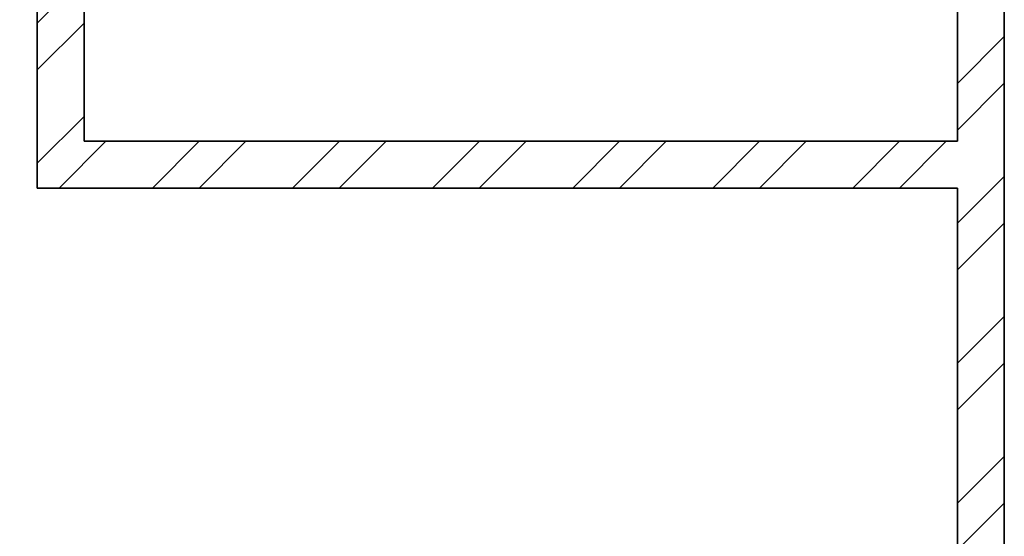
# Model space of a CAD drawing. Units: inches. Extents: x 1885 to 2748, y 783 to 2421.
# Tile 110 of 117: x 2524 to 2618, y 1977 to 2027. Entities that reach past the tile are written whole.
import ezdxf

# ---------------------------------------------------------------- set-up
doc = ezdxf.new("R2010")
doc.units = ezdxf.units.IN
doc.layers.add('A-WALL', color=7, linetype='Continuous', lineweight=35)
doc.layers.add('A-WALL-PATT', color=85, linetype='Continuous', lineweight=13, true_color=0x58ba48)

msp = doc.modelspace()

# ---------------------------------------------------------------- hatches: boundary and pattern name
at = {"layer": 'A-WALL-PATT'}
h = msp.add_hatch(dxfattribs=at)
h.set_pattern_fill('ANSI32', color=256)
h.paths.add_polyline_path([(2007.772, 2318.006), (1980.774, 2318.006), (1980.774, 2281.215), (1985.274, 2281.215), (1985.274, 2313.506), (2007.772, 2313.506), (2007.772, 2315.756)])
h.paths.add_polyline_path([(2094.324, 2318.006), (2067.772, 2318.006), (2067.772, 2313.506), (2094.324, 2313.506), (2094.324, 2315.756)])
h.paths.add_polyline_path([(2131.367, 2315.756), (2131.367, 2318.006), (2131.189, 2318.006), (2112.609, 2318.006), (2112.609, 2313.506), (2117.274, 2313.506), (2117.274, 2255.201), (2121.774, 2255.201), (2121.774, 2313.506), (2131.367, 2313.506)])
h.paths.add_polyline_path([(2190.512, 2318.006), (2155.367, 2318.006), (2155.367, 2313.506), (2169.774, 2313.506), (2169.774, 2229.506), (2121.774, 2229.506), (2121.774, 2233.451), (2119.524, 2233.451), (2117.274, 2233.451), (2117.274, 2201.101), (2121.774, 2201.101), (2121.774, 2225.006), (2169.774, 2225.006), (2169.774, 2165.006), (2306.274, 2165.006), (2306.274, 2066.006), (2310.774, 2066.006), (2344.274, 2066.006), (2486.274, 2066.006), (2486.274, 1886.006), (2483.02, 1886.006), (2483.02, 1881.506), (2486.274, 1881.506), (2486.274, 1880.678), (2490.774, 1880.678), (2490.774, 2070.506), (2344.274, 2070.506), (2310.774, 2070.506), (2310.774, 2165.006), (2310.774, 2173.636), (2308.524, 2173.636), (2306.274, 2173.636), (2306.274, 2169.506), (2174.274, 2169.506), (2174.274, 2313.506), (2190.512, 2313.506), (2190.512, 2315.756)])
h.paths.add_polyline_path([(1985.274, 2221.215), (1980.774, 2221.215), (1980.774, 2165.006), (1992.774, 2165.006), (1992.774, 2141.927), (1997.274, 2141.927), (1997.274, 2165.006), (2117.274, 2165.006), (2117.274, 2163.126), (2121.774, 2163.126), (2121.774, 2172.734), (2119.524, 2172.734), (2117.274, 2172.734), (2117.274, 2169.506), (1985.274, 2169.506)])
h.paths.add_polyline_path([(1997.274, 2105.927), (1992.774, 2105.927), (1992.774, 2070.506), (2016.774, 2070.506), (2016.774, 2059.123), (2019.024, 2059.123), (2021.274, 2059.123), (2021.274, 2070.506), (2117.274, 2070.506), (2117.274, 2022.506), (2114.423, 2022.506), (2114.423, 2018.006), (2123.627, 2018.006), (2123.627, 2020.256), (2123.627, 2022.506), (2121.774, 2022.506), (2121.774, 2142.587), (2119.524, 2142.587), (2117.274, 2142.587), (2117.274, 2075.006), (1997.274, 2075.006)])
h.paths.add_polyline_path([(2092.029, 2020.256), (2092.029, 2022.506), (2021.274, 2022.506), (2021.274, 2035.123), (2016.774, 2035.123), (2016.774, 2018.006), (2016.774, 1978.784), (2021.274, 1978.784), (2021.274, 2018.006), (2092.029, 2018.006)])
h.paths.add_polyline_path([(2260.938, 2022.506), (2153.105, 2022.506), (2153.105, 2020.256), (2153.105, 2018.006), (2155.274, 2018.006), (2155.274, 1886.006), (2107.629, 1886.006), (2107.629, 1881.506), (2182.911, 1881.506), (2182.911, 1883.756), (2182.911, 1886.006), (2159.774, 1886.006), (2159.774, 2018.006), (2260.938, 2018.006), (2260.938, 2020.256)])
h.paths.add_polyline_path([(2047.629, 1883.756), (2047.629, 1886.006), (2021.274, 1886.006), (2021.274, 1918.784), (2019.024, 1918.784), (2016.774, 1918.784), (2016.774, 1881.506), (2047.629, 1881.506)])
h.paths.add_polyline_path([(2306.361, 1883.756), (2306.361, 1886.006), (2296.274, 1886.006), (2296.274, 1982.006), (2316.535, 1982.006), (2316.535, 1984.256), (2316.535, 1986.506), (2296.274, 1986.506), (2296.274, 2022.506), (2289.276, 2022.506), (2289.276, 2018.006), (2291.774, 2018.006), (2291.774, 1886.006), (2242.911, 1886.006), (2242.911, 1881.506), (2306.361, 1881.506)], flags=17)
h.paths.add_polyline_path([(1985.274, 1843.006), (2021.6, 1843.006), (2021.534, 1845.441), (2021.477, 1847.506), (1980.774, 1847.506), (1980.774, 1809.446), (1985.274, 1809.446)])
h.paths.add_polyline_path([(2131.482, 1845.256), (2131.482, 1847.506), (2081.534, 1847.506), (2081.534, 1843.006), (2117.274, 1843.006), (2117.274, 1784.147), (2119.524, 1784.147), (2121.774, 1784.147), (2121.774, 1843.006), (2131.482, 1843.006)])
h.paths.add_polyline_path([(2203.886, 1847.506), (2155.482, 1847.506), (2155.482, 1843.006), (2169.774, 1843.006), (2169.774, 1759.006), (2121.774, 1759.006), (2121.774, 1761.457), (2117.274, 1761.457), (2117.274, 1730.429), (2121.774, 1730.429), (2121.774, 1754.506), (2177.421, 1754.506), (2177.421, 1756.756), (2177.421, 1759.006), (2174.274, 1759.006), (2174.274, 1843.006), (2203.886, 1843.006)])
h.paths.add_polyline_path([(2335.554, 1845.256), (2335.554, 1847.506), (2239.886, 1847.506), (2239.886, 1843.006), (2306.274, 1843.006), (2306.274, 1759.006), (2199.486, 1759.006), (2199.486, 1754.506), (2310.774, 1754.506), (2310.774, 1843.006), (2335.554, 1843.006)])
h.paths.add_polyline_path([(2348.774, 2022.506), (2344.274, 2022.506), (2344.274, 1986.506), (2341.681, 1986.506), (2341.681, 1982.006), (2344.274, 1982.006), (2344.274, 1886.006), (2330.361, 1886.006), (2330.361, 1881.506), (2361.627, 1881.506), (2361.627, 1883.756), (2361.627, 1886.006), (2348.774, 1886.006)], flags=17)
h.paths.add_polyline_path([(2283.251, 2315.756), (2283.251, 2318.006), (2238.512, 2318.006), (2238.512, 2313.506), (2283.251, 2313.506)], flags=17)
h.paths.add_polyline_path([(2363.274, 2348.006), (2388.677, 2348.006), (2388.677, 2350.256), (2388.677, 2352.506), (2358.774, 2352.506), (2358.774, 2348.006), (2358.774, 2318.006), (2344.481, 2318.006), (2344.481, 2313.506), (2358.774, 2313.506), (2358.774, 2229.506), (2310.774, 2229.506), (2310.774, 2231.952), (2306.274, 2231.952), (2306.274, 2205.611), (2310.774, 2205.611), (2310.774, 2225.006), (2358.774, 2225.006), (2358.774, 2211.506), (2452.329, 2211.506), (2452.329, 2213.756), (2452.329, 2216.006), (2363.274, 2216.006), (2363.274, 2318.006)])
h.paths.add_polyline_path([(2310.774, 2313.506), (2320.481, 2313.506), (2320.481, 2315.756), (2320.481, 2318.006), (2302.728, 2318.006), (2302.728, 2313.506), (2306.274, 2313.506), (2306.274, 2251.076), (2310.774, 2251.076)], flags=17)
h.paths.add_polyline_path([(2490.774, 2352.506), (2486.274, 2352.506), (2448.677, 2352.506), (2448.677, 2348.006), (2486.274, 2348.006), (2486.274, 2318.006), (2486.274, 2216.006), (2481.78, 2216.006), (2481.78, 2211.506), (2486.274, 2211.506), (2486.274, 2165.006), (2493.289, 2165.006), (2493.289, 2167.256), (2493.289, 2169.506), (2490.774, 2169.506), (2490.774, 2313.506), (2494.429, 2313.506), (2494.429, 2318.006), (2490.774, 2318.006)])
h.paths.add_polyline_path([(2534.653, 2318.006), (2515.691, 2318.006), (2515.691, 2313.506), (2534.653, 2313.506), (2534.653, 2315.756)])
h.paths.add_polyline_path([(2618.274, 2318.006), (2594.653, 2318.006), (2594.653, 2313.506), (2613.774, 2313.506), (2613.774, 2281.706), (2618.274, 2281.706)])
h.paths.add_polyline_path([(2618.274, 2221.706), (2613.774, 2221.706), (2613.774, 2169.506), (2554.019, 2169.506), (2554.019, 2165.006), (2613.774, 2165.006), (2613.774, 2152.878), (2618.274, 2152.878)])
h.paths.add_polyline_path([(2618.274, 2128.878), (2616.024, 2128.878), (2613.774, 2128.878), (2613.774, 2117.006), (2529.774, 2117.006), (2529.774, 2165.006), (2532.848, 2165.006), (2532.848, 2169.506), (2522.867, 2169.506), (2522.867, 2165.006), (2525.274, 2165.006), (2525.274, 2117.006), (2525.274, 2112.506), (2525.274, 2108.576), (2529.774, 2108.576), (2529.774, 2112.506), (2613.774, 2112.506), (2613.774, 2080.19), (2618.274, 2080.19)])
h.paths.add_polyline_path([(2618.274, 2044.19), (2616.024, 2044.19), (2613.774, 2044.19), (2613.774, 2015.506), (2529.774, 2015.506), (2529.774, 2088.582), (2527.524, 2088.582), (2525.274, 2088.582), (2525.274, 2011.006), (2613.774, 2011.006), (2613.774, 1956.755), (2618.274, 1956.755)])
h.paths.add_polyline_path([(2618.274, 1881.506), (2618.274, 1896.755), (2613.774, 1896.755), (2613.774, 1881.506), (2613.774, 1847.506), (2592.715, 1847.506), (2592.715, 1843.006), (2613.774, 1843.006), (2613.774, 1765.006), (2613.774, 1760.506), (2609.621, 1760.506), (2609.621, 1756.006), (2613.774, 1756.006), (2613.774, 1660.006), (2608.544, 1660.006), (2608.544, 1655.506), (2613.774, 1655.506), (2613.774, 1508.158), (2618.274, 1508.158)])
h.paths.add_polyline_path([(2565.774, 1843.006), (2568.997, 1843.006), (2568.997, 1847.506), (2490.774, 1847.506), (2490.774, 1849.7), (2488.524, 1849.7), (2486.274, 1849.7), (2486.274, 1847.506), (2477.274, 1847.506), (2477.274, 1838.506), (2477.274, 1821.493), (2486.274, 1821.493), (2486.274, 1838.506), (2561.274, 1838.506), (2561.274, 1765.006), (2486.274, 1765.006), (2486.274, 1786.157), (2477.274, 1786.157), (2477.274, 1765.006), (2477.274, 1756.006), (2486.274, 1756.006), (2565.774, 1756.006), (2585.621, 1756.006), (2585.621, 1758.256), (2585.621, 1760.506), (2565.774, 1760.506), (2565.774, 1765.006)])
h.paths.add_polyline_path([(2486.274, 1651.006), (2561.274, 1651.006), (2561.274, 1567.006), (2486.274, 1567.006), (2486.274, 1591.321), (2477.274, 1591.321), (2477.274, 1567.006), (2477.274, 1558.006), (2477.274, 1555.439), (2481.774, 1555.439), (2481.774, 1558.006), (2568.653, 1558.006), (2568.653, 1560.256), (2568.653, 1562.506), (2565.774, 1562.506), (2565.774, 1655.506), (2584.544, 1655.506), (2584.544, 1657.756), (2584.544, 1660.006), (2565.774, 1660.006), (2486.274, 1660.006), (2477.274, 1660.006), (2477.274, 1651.006), (2477.274, 1632.989), (2486.274, 1632.989)])
h.paths.add_polyline_path([(2449.967, 1883.756), (2449.967, 1886.006), (2421.627, 1886.006), (2421.627, 1881.506), (2449.967, 1881.506)], flags=17)
h.paths.add_polyline_path([(2447.274, 1847.506), (2395.554, 1847.506), (2395.554, 1843.006), (2442.774, 1843.006), (2442.774, 1809.27), (2447.274, 1809.27)])
h.paths.add_polyline_path([(1985.274, 1749.446), (1980.774, 1749.446), (1980.774, 1694.504), (1985.274, 1694.504), (1985.274, 1694.506), (1986.897, 1694.506), (1986.897, 1697.78), (1986.897, 1699.006), (1985.274, 1699.006)])
h.paths.add_polyline_path([(2152.774, 1699.006), (2121.774, 1699.006), (2121.774, 1703.668), (2119.524, 1703.668), (2117.274, 1703.668), (2117.274, 1699.006), (2009.219, 1699.006), (2009.219, 1694.506), (2148.274, 1694.506), (2148.274, 1692.631), (2152.774, 1692.631)])
h.paths.add_polyline_path([(2016.274, 1694.506), (2011.774, 1694.506), (2011.774, 1558.006), (2040.806, 1558.006), (2040.806, 1560.256), (2040.806, 1562.506), (2016.274, 1562.506)])
h.paths.add_polyline_path([(2152.774, 1663.017), (2150.524, 1663.017), (2148.274, 1663.017), (2148.274, 1562.506), (2100.806, 1562.506), (2100.806, 1558.006), (2165.119, 1558.006), (2165.119, 1560.256), (2165.119, 1562.506), (2152.774, 1562.506), (2152.774, 1610.506), (2224.774, 1610.506), (2224.774, 1607.99), (2229.274, 1607.99), (2229.274, 1615.006), (2152.774, 1615.006)])
h.paths.add_polyline_path([(2238.613, 1560.256), (2238.613, 1562.506), (2229.274, 1562.506), (2229.274, 1588.756), (2227.024, 1588.763), (2224.774, 1588.771), (2224.774, 1562.506), (2189.119, 1562.506), (2189.119, 1558.006), (2238.613, 1558.006)])
h.paths.add_polyline_path([(2336.024, 1560.256), (2336.024, 1562.506), (2310.774, 1562.506), (2310.774, 1656.347), (2308.524, 1656.347), (2306.274, 1656.347), (2306.274, 1562.506), (2286.613, 1562.506), (2286.613, 1558.006), (2336.024, 1558.006)])
h.paths.add_polyline_path([(2447.274, 1690.968), (2445.024, 1690.968), (2442.774, 1690.968), (2442.774, 1687.006), (2306.274, 1687.006), (2306.274, 1680.75), (2310.774, 1680.75), (2310.774, 1682.506), (2442.774, 1682.506), (2442.774, 1562.506), (2396.024, 1562.506), (2396.024, 1558.006), (2447.274, 1558.006)])
h.paths.add_polyline_path([(2447.274, 1749.27), (2445.024, 1749.27), (2442.774, 1749.27), (2442.774, 1717.232), (2447.274, 1717.232)])
h.paths.add_polyline_path([(2044.674, 1521.756), (2044.674, 1524.006), (2007.274, 1524.006), (2007.274, 1503.49), (2009.524, 1503.49), (2011.774, 1503.49), (2011.774, 1519.506), (2044.674, 1519.506)])
h.paths.add_polyline_path([(2177.969, 1521.756), (2177.969, 1524.006), (2104.674, 1524.006), (2104.674, 1519.506), (2145.774, 1519.506), (2145.774, 1387.506), (2143.37, 1387.506), (2143.37, 1383.006), (2251.585, 1383.006), (2251.585, 1385.256), (2251.585, 1387.506), (2150.274, 1387.506), (2150.274, 1519.506), (2177.969, 1519.506)])
h.paths.add_polyline_path([(2298.704, 1524.006), (2237.969, 1524.006), (2237.969, 1519.506), (2282.274, 1519.506), (2282.274, 1387.506), (2279.683, 1387.506), (2279.683, 1383.006), (2286.774, 1383.006), (2286.774, 1419.006), (2312.451, 1419.006), (2312.451, 1421.256), (2312.451, 1423.506), (2286.774, 1423.506), (2286.774, 1519.506), (2298.704, 1519.506), (2298.704, 1521.722)], flags=17)
h.paths.add_polyline_path([(2361.897, 1521.756), (2361.897, 1524.006), (2322.704, 1524.006), (2322.704, 1519.506), (2334.774, 1519.506), (2334.774, 1423.506), (2331.93, 1423.506), (2331.93, 1419.006), (2334.774, 1419.006), (2334.774, 1387.506), (2334.774, 1383.228), (2339.274, 1383.228), (2339.274, 1387.506), (2339.274, 1519.506), (2361.897, 1519.506)], flags=17)
h.paths.add_polyline_path([(2447.274, 1521.756), (2447.274, 1524.006), (2421.897, 1524.006), (2421.897, 1519.506), (2447.274, 1519.506)], flags=17)
h.paths.add_polyline_path([(2481.774, 1529.6), (2479.524, 1529.6), (2477.274, 1529.6), (2477.274, 1524.006), (2474.489, 1524.006), (2474.489, 1519.506), (2477.274, 1519.506), (2477.274, 1334.506), (2296.774, 1334.506), (2296.774, 1240.506), (2160.274, 1240.506), (2160.274, 1180.506), (2112.274, 1180.506), (2112.274, 1207.692), (2110.024, 1207.692), (2107.774, 1207.692), (2107.774, 1171.609), (2112.274, 1171.609), (2112.274, 1176.006), (2160.274, 1176.006), (2160.274, 1092.006), (2144.221, 1092.006), (2144.221, 1087.506), (2189.497, 1087.506), (2189.497, 1089.756), (2189.497, 1092.006), (2164.774, 1092.006), (2164.774, 1236.006), (2296.774, 1236.006), (2296.774, 1231.912), (2301.274, 1231.912), (2301.274, 1330.006), (2481.774, 1330.006), (2481.774, 1387.506)])
h.paths.add_polyline_path([(2618.274, 1448.158), (2613.774, 1448.158), (2613.774, 1382.506), (2529.774, 1382.506), (2525.274, 1382.506), (2525.274, 1307.062), (2529.774, 1307.062), (2529.774, 1378.006), (2613.774, 1378.006), (2613.774, 1354.988), (2618.274, 1354.988)])
h.paths.add_polyline_path([(2618.274, 1318.988), (2613.774, 1318.988), (2613.774, 1281.006), (2529.774, 1281.006), (2529.774, 1283.786), (2527.524, 1283.786), (2525.274, 1283.786), (2525.274, 1228.506), (2516.794, 1228.506), (2516.794, 1224.006), (2533.484, 1224.006), (2533.484, 1226.256), (2533.484, 1228.506), (2529.774, 1228.506), (2529.774, 1276.506), (2613.774, 1276.506), (2613.774, 1266.02), (2618.274, 1266.02)])
h.paths.add_polyline_path([(2618.274, 1134.964), (2613.774, 1134.964), (2613.774, 1092.006), (2594.545, 1092.006), (2594.545, 1087.506), (2618.274, 1087.506)])
h.paths.add_polyline_path([(2534.545, 1092.006), (2509.765, 1092.006), (2509.765, 1087.506), (2534.545, 1087.506), (2534.545, 1089.756)])
h.paths.add_polyline_path([(2481.274, 1224.006), (2484.117, 1224.006), (2484.117, 1226.256), (2484.117, 1228.506), (2476.774, 1228.506), (2476.774, 1198.506), (2471.61, 1198.506), (2471.61, 1194.006), (2476.774, 1194.006), (2476.774, 1062.006), (2436.894, 1062.006), (2436.894, 1057.506), (2476.774, 1057.506), (2481.274, 1057.506), (2481.274, 1062.006), (2481.274, 1087.506), (2485.354, 1087.506), (2485.354, 1089.756), (2485.354, 1092.006), (2481.274, 1092.006), (2481.274, 1117.506)])
h.paths.add_polyline_path([(2439.898, 1198.506), (2349.274, 1198.506), (2349.274, 1194.006), (2349.274, 1180.506), (2301.274, 1180.506), (2301.274, 1201.896), (2299.024, 1201.896), (2296.774, 1201.896), (2296.774, 1172.335), (2299.024, 1172.335), (2301.274, 1172.335), (2301.274, 1176.006), (2349.274, 1176.006), (2349.274, 1092.006), (2334.452, 1092.006), (2334.452, 1087.506), (2349.274, 1087.506), (2349.274, 1057.506), (2353.774, 1057.506), (2376.894, 1057.506), (2376.894, 1059.756), (2376.894, 1062.006), (2353.774, 1062.006), (2353.774, 1087.506), (2353.774, 1180.506), (2353.774, 1194.006), (2439.898, 1194.006), (2439.898, 1196.256)])
h.paths.add_polyline_path([(2270.596, 1089.756), (2270.596, 1092.006), (2249.497, 1092.006), (2249.497, 1087.506), (2270.596, 1087.506)], flags=17)
h.paths.add_polyline_path([(2310.452, 1092.006), (2301.274, 1092.006), (2301.274, 1153.292), (2296.774, 1153.292), (2296.774, 1092.006), (2293.786, 1092.006), (2293.786, 1087.506), (2310.452, 1087.506), (2310.452, 1089.756)], flags=17)
h.paths.add_polyline_path([(2112.274, 1150.328), (2110.024, 1150.328), (2107.774, 1150.328), (2107.774, 1092.006), (2104.465, 1092.006), (2104.465, 1087.506), (2120.221, 1087.506), (2120.221, 1089.756), (2120.221, 1092.006), (2112.274, 1092.006)])
h.paths.add_polyline_path([(2082.172, 1092.006), (2058.144, 1092.006), (2058.144, 1087.506), (2082.172, 1087.506), (2082.172, 1089.756)])
h.paths.add_polyline_path([(1975.774, 1145.638), (1971.274, 1145.638), (1971.274, 1087.506), (1980.774, 1087.506), (1998.144, 1087.506), (1998.144, 1089.756), (1998.144, 1092.006), (1985.274, 1092.006), (1975.774, 1092.006)])
h.paths.add_polyline_path([(2112.274, 1244.385), (2110.024, 1244.385), (2107.774, 1244.385), (2107.774, 1240.506), (1992.274, 1240.506), (1992.274, 1271.008), (1987.774, 1271.008), (1987.774, 1240.506), (1980.774, 1240.506), (1975.774, 1240.506), (1971.274, 1240.506), (1971.274, 1205.638), (1975.774, 1205.638), (1975.774, 1236.006), (2107.774, 1236.006), (2107.774, 1233.444), (2112.274, 1233.444), (2112.274, 1236.006)])
h.paths.add_polyline_path([(2112.274, 1383.006), (2114.783, 1383.006), (2114.783, 1385.256), (2114.783, 1387.506), (2102.476, 1387.506), (2102.476, 1383.006), (2107.774, 1383.006), (2107.774, 1335.006), (2011.774, 1335.006), (2011.774, 1349.939), (2007.274, 1349.939), (2007.274, 1335.006), (1987.774, 1335.006), (1987.774, 1330.506), (1987.774, 1307.008), (1992.274, 1307.008), (1992.274, 1330.506), (2007.274, 1330.506), (2107.774, 1330.506), (2107.774, 1264.711), (2112.274, 1264.711)])
h.paths.add_polyline_path([(2077.857, 1387.506), (2011.774, 1387.506), (2011.774, 1390.036), (2009.524, 1390.036), (2007.274, 1390.036), (2007.274, 1373.939), (2011.774, 1373.939), (2011.774, 1383.006), (2077.857, 1383.006)])
h.paths.add_polyline_path([(2011.774, 1443.49), (2007.274, 1443.49), (2007.274, 1410.248), (2011.774, 1410.248)])

# ---------------------------------------------------------------- linework, layer by layer
at = {"layer": 'A-WALL'}
for p, q in [((2529.774, 2089.82), (2529.774, 2015.506)), ((2525.274, 2088.582), (2525.274, 2011.006)), ((2613.774, 2044.19), (2613.774, 2015.506)), ((2618.274, 2044.19), (2618.274, 1956.755)), ((2529.774, 2015.506), (2613.774, 2015.506)), ((2525.274, 2011.006), (2613.774, 2011.006)), ((2613.774, 2011.006), (2613.774, 1956.755))]:
    msp.add_line(p, q, dxfattribs=at)

doc.saveas('drawing.dxf')
